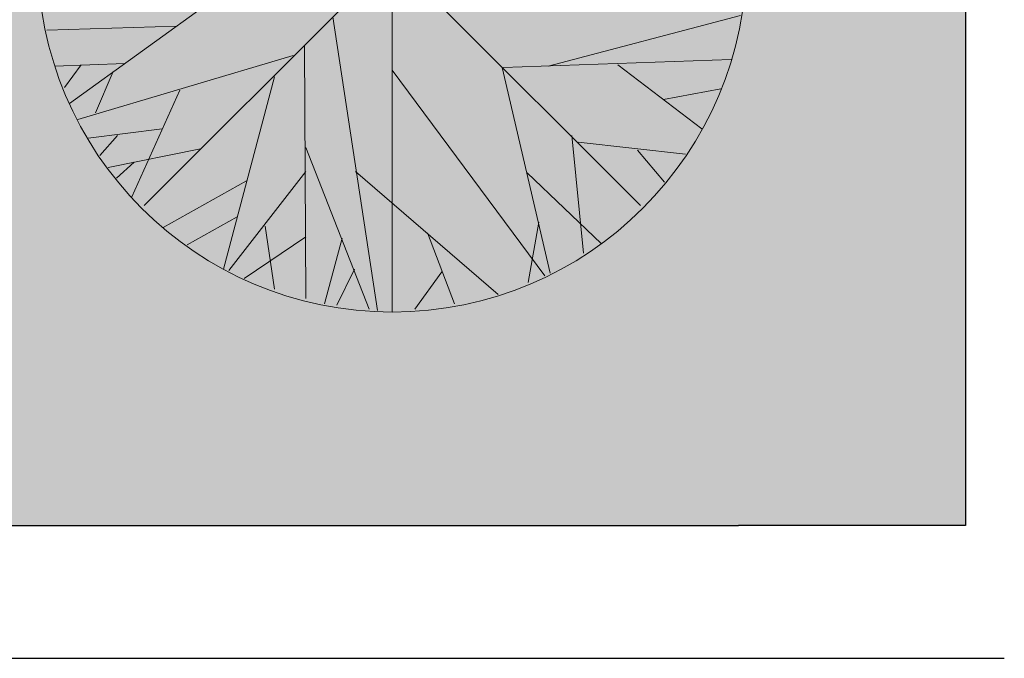
# Model space of a CAD drawing. Units: inches. Extents: x 459864 to 460310, y 324185 to 324787.
# Tile 73 of 112: x 460238 to 460271, y 324195 to 324217. Entities that reach past the tile are written whole.
import ezdxf

# ---------------------------------------------------------------- set-up
doc = ezdxf.new("R2010")
doc.units = ezdxf.units.IN
for name, color, linetype, lineweight in [('A-ANNO-DIMS', 2, 'Continuous', 18), ('C-PROP', 7, 'Continuous', 30), ('L-PLNT', 3, 'Continuous', 13), ('L-SITE-PATT', 252, 'Continuous', 13)]:
    doc.layers.add(name, color=color, linetype=linetype, lineweight=lineweight)
doc.styles.get("Standard").update_dxf_attribs({"font": 'arial.ttf'})
doc.dimstyles.new('ISO-25', dxfattribs={"dimtxt": 6, "dimasz": 2.5, "dimexe": 1.25, "dimexo": 0.625, "dimtad": 1, "dimdec": 1, "dimlunit": 3, "dimtxsty": 'Standard', "dimcen": 2.5, "dimadec": 0, "dimazin": 0, "dimtfac": 1, "dimtdec": 1, "dimtmove": 0, "dimatfit": 3, "dimfxl": 1, "dimarcsym": 0})

# ---------------------------------------------------------------- blocks, each defined once
blk = doc.blocks.new('Tree - deciduous plan')
for p, q in [((0, 59.9996), (0, -60)), ((42, 42), (-42, -42)), ((42, -42), (-42, 42)), ((-54.6162, -24.7335), (-20.2853, 0.0941)), ((26.3697, -18.4138), (58.9401, -9.8369)), ((-58.4895, -12.3197), (-36.4825, -11.6426)), ((-10.074, -10.0627), (-2.5036, -59.7178)), ((-53.2078, -27.442), (-16.7641, -16.6081)), ((-14.8275, -15.0282), (-14.6515, -57.6865)), ((-57.081, -18.4138), (-45.2853, -17.9624)), ((-52.6797, -18.188), (-55.4966, -22.0251)), ((18.7992, -18.6394), (57.3556, -17.2853)), ((38.1654, -18.188), (52.426, -29.0219)), ((-47.2219, -19.3166), (-50.2148, -26.3135)), ((-0.0388, -19.0909), (25.8415, -53.8495)), ((18.6232, -18.6394), (26.7218, -53.3981)), ((-19.9331, -20.2194), (-28.5599, -52.721)), ((-35.9543, -22.4765), (-44.0529, -40.5329)), ((45.9119, -24.0564), (55.595, -22.2508)), ((-38.9472, -29.0219), (-51.4472, -30.6018)), ((-46.5177, -30.1504), (-49.5106, -33.536)), ((30.419, -30.1504), (32.3556, -50.0125)), ((31.4753, -31.279), (49.6091, -33.3103)), ((-32.4331, -32.4075), (-48.1021, -35.5674)), ((-14.6515, -32.1818), (-3.912, -59.4922)), ((41.5105, -32.6332), (46.088, -38.0501)), ((-43.7008, -34.6645), (-46.6937, -37.373)), ((-14.6515, -36.2445), (-27.6797, -52.9467)), ((-6.2008, -36.2445), (17.919, -57.0094)), ((22.8485, -36.4702), (35.3485, -48.4326)), ((-24.6867, -37.8244), (-38.7712, -45.7241)), ((-26.2712, -43.9185), (-34.7219, -48.6583)), ((24.7852, -44.8213), (23.0246, -54.978)), ((-21.5177, -45.4984), (-19.9331, -56.1065)), ((5.9471, -46.6269), (10.5246, -58.5893)), ((-14.6515, -47.3041), (-25.0388, -54.3009)), ((-8.4895, -47.5298), (-11.4825, -58.5893)), ((-6.3768, -52.721), (-9.3698, -58.815)), ((8.4119, -53.1724), (3.8344, -59.4922))]:
    blk.add_line(p, q)
blk.add_circle((0, 0), 60)
blk = doc.blocks.new('*D65')
at = {"layer": 'A-ANNO-DIMS', "color": 0, "lineweight": -2, "transparency": 16777216}
for p, q in [((460247.74, 324283.483), (460302.765, 324283.483)), ((460301.515, 324280.983), (460301.515, 324197.483)), ((460271.74, 324194.983), (460302.765, 324194.983))]:
    blk.add_line(p, q, dxfattribs=at)
at = {"layer": 'A-ANNO-DIMS', "color": 0, "transparency": 16777216}
for points in [[(460301.098, 324280.983), (460301.932, 324280.983), (460301.515, 324283.483)], [(460301.098, 324197.483), (460301.932, 324197.483), (460301.515, 324194.983)]]:
    blk.add_solid(points, dxfattribs=at)
at = {"layer": 'Defpoints', "color": 0, "transparency": 16777216}
for p in [(460247.115, 324283.483), (460271.115, 324194.983), (460301.515, 324194.983)]:
    blk.add_point(p, dxfattribs=at)
at = {"layer": 'A-ANNO-DIMS', "color": 0, "transparency": 16777216, "insert": (460297.788, 324239.233), "char_height": 6, "attachment_point": 5, "rotation": 90}
blk.add_mtext('7\'-4 1/2"', dxfattribs=at)

msp = doc.modelspace()

# ---------------------------------------------------------------- hatches: boundary and pattern name
at = {"layer": 'L-SITE-PATT'}
h = msp.add_hatch(dxfattribs=at)
h.set_pattern_fill('DOTS', color=256)
h.paths.add_polyline_path([(460269.804, 324283.483), (460247.115, 324283.483), (460121.929, 324283.483), (460121.929, 324252.473), (460117.429, 324252.473), (460110.124, 324252.473), (460110.124, 324243.287), (460080.83, 324243.287), (460080.83, 324252.473), (460061.115, 324252.473), (460061.115, 324251.882), (460077.909, 324251.882), (460077.909, 324199.483), (460080.83, 324199.483), (460080.83, 324207.553), (460110.124, 324207.553), (460110.124, 324199.483), (460110.813, 324199.483), (460262.115, 324199.483), (460269.804, 324199.483)], flags=17)
edge = h.paths.add_edge_path(flags=0)
edge.add_ellipse((460222.59, 324263.813), major_axis=(-8.485, 8.485), ratio=1, start_angle=405, end_angle=495, ccw=False)
edge.add_line((460214.821, 324254.66), (460214.832, 324254.666))
edge.add_ellipse((460222.59, 324263.813), major_axis=(-8.485, 8.485), ratio=1, start_angle=405, end_angle=495, ccw=False)
edge.add_line((460210.759, 324261.781), (460210.768, 324261.787))
edge.add_ellipse((460222.59, 324263.813), major_axis=(-8.485, 8.485), ratio=1, start_angle=405, end_angle=495, ccw=False)
edge.add_ellipse((460222.59, 324263.813), major_axis=(-8.485, 8.485), ratio=1, start_angle=392.754, end_angle=405, ccw=False)
edge.add_ellipse((460222.59, 324263.813), major_axis=(-8.485, 8.485), ratio=1, start_angle=380.9347, end_angle=392.754, ccw=False)
edge.add_line((460211.337, 324267.985), (460211.34, 324267.985))
edge.add_ellipse((460222.59, 324263.813), major_axis=(-8.485, 8.485), ratio=1, start_angle=380.9347, end_angle=392.754, ccw=False)
edge.add_ellipse((460222.59, 324263.813), major_axis=(-8.485, 8.485), ratio=1, start_angle=347.9015, end_angle=380.9347, ccw=False)
edge.add_ellipse((460222.59, 324263.813), major_axis=(-8.485, 8.485), ratio=1, start_angle=327.0619, end_angle=347.9015, ccw=False)
edge.add_ellipse((460222.59, 324263.813), major_axis=(-8.485, 8.485), ratio=1, start_angle=278.3246, end_angle=327.0619, ccw=False)
edge.add_line((460225.158, 324275.536), (460225.158, 324275.535))
edge.add_ellipse((460222.59, 324263.813), major_axis=(-8.485, 8.485), ratio=1, start_angle=278.3246, end_angle=327.0619, ccw=False)
edge.add_ellipse((460222.59, 324263.813), major_axis=(-8.485, 8.485), ratio=1, start_angle=260.6436, end_angle=278.3246, ccw=False)
edge.add_ellipse((460222.59, 324263.813), major_axis=(-8.485, 8.485), ratio=1, start_angle=225, end_angle=260.6436, ccw=False)
edge.add_line((460234.509, 324265.243), (460234.501, 324265.239))
edge.add_ellipse((460222.59, 324263.813), major_axis=(-8.485, 8.485), ratio=1, start_angle=225, end_angle=260.6436, ccw=False)
edge.add_ellipse((460222.59, 324263.813), major_axis=(-8.485, 8.485), ratio=1, start_angle=495, end_angle=585, ccw=False)
edge.add_line((460234.437, 324261.861), (460234.424, 324261.858))
edge.add_ellipse((460222.59, 324263.813), major_axis=(-8.485, 8.485), ratio=1, start_angle=495, end_angle=585, ccw=False)
edge.add_line((460227.95, 324253.067), (460227.946, 324253.083))
edge.add_ellipse((460222.59, 324263.813), major_axis=(-8.485, 8.485), ratio=1, start_angle=495, end_angle=585, ccw=False)
edge.add_line((460226.223, 324252.369), (460226.211, 324252.38))
edge.add_ellipse((460222.59, 324263.813), major_axis=(-8.485, 8.485), ratio=1, start_angle=495, end_angle=585, ccw=False)
h.paths.add_polyline_path([(460219.651, 324254.347), (460218.461, 324253.545), (460218.275, 324254.789), (460219.642, 324256.542), (460219.625, 324260.848), (460216.11, 324257.333), (460214.35, 324256.978), (460215.416, 324259.356), (460212.524, 324258.496), (460213.137, 324259.93), (460218.507, 324263.813), (460222.59, 324263.813), (460222.59, 324267.807), (460218.176, 324272.212), (460219.026, 324274.639), (460222.59, 324272.811), (460222.59, 324275.423), (460223.057, 324274.825), (460222.675, 324273.492), (460225.912, 324267.135), (460219.625, 324260.848)], flags=0)
edge = h.paths.add_edge_path(flags=0)
edge.add_ellipse((460194.576, 324264.046), major_axis=(-8.485, 8.485), ratio=1, start_angle=495, end_angle=585, ccw=False)
edge.add_line((460199.936, 324253.3), (460199.932, 324253.316))
edge.add_ellipse((460194.576, 324264.046), major_axis=(-8.485, 8.485), ratio=1, start_angle=495, end_angle=585, ccw=False)
edge.add_line((460198.208, 324252.603), (460198.196, 324252.613))
edge.add_ellipse((460194.576, 324264.046), major_axis=(-8.485, 8.485), ratio=1, start_angle=495, end_angle=585, ccw=False)
edge.add_ellipse((460194.576, 324264.046), major_axis=(-8.485, 8.485), ratio=1, start_angle=405, end_angle=495, ccw=False)
edge.add_line((460186.806, 324254.893), (460186.817, 324254.899))
edge.add_ellipse((460194.576, 324264.046), major_axis=(-8.485, 8.485), ratio=1, start_angle=405, end_angle=495, ccw=False)
edge.add_line((460182.744, 324262.014), (460182.753, 324262.02))
edge.add_ellipse((460194.576, 324264.046), major_axis=(-8.485, 8.485), ratio=1, start_angle=405, end_angle=495, ccw=False)
edge.add_ellipse((460194.576, 324264.046), major_axis=(-8.485, 8.485), ratio=1, start_angle=392.754, end_angle=405, ccw=False)
edge.add_ellipse((460194.576, 324264.046), major_axis=(-8.485, 8.485), ratio=1, start_angle=380.9347, end_angle=392.754, ccw=False)
edge.add_line((460183.323, 324268.218), (460183.326, 324268.218))
edge.add_ellipse((460194.576, 324264.046), major_axis=(-8.485, 8.485), ratio=1, start_angle=380.9347, end_angle=392.754, ccw=False)
edge.add_ellipse((460194.576, 324264.046), major_axis=(-8.485, 8.485), ratio=1, start_angle=347.9015, end_angle=380.9347, ccw=False)
edge.add_ellipse((460194.576, 324264.046), major_axis=(-8.485, 8.485), ratio=1, start_angle=327.0619, end_angle=347.9015, ccw=False)
edge.add_ellipse((460194.576, 324264.046), major_axis=(-8.485, 8.485), ratio=1, start_angle=278.3246, end_angle=327.0619, ccw=False)
edge.add_line((460197.144, 324275.769), (460197.143, 324275.768))
edge.add_ellipse((460194.576, 324264.046), major_axis=(-8.485, 8.485), ratio=1, start_angle=278.3246, end_angle=327.0619, ccw=False)
edge.add_ellipse((460194.576, 324264.046), major_axis=(-8.485, 8.485), ratio=1, start_angle=260.6436, end_angle=278.3246, ccw=False)
edge.add_ellipse((460194.576, 324264.046), major_axis=(-8.485, 8.485), ratio=1, start_angle=225, end_angle=260.6436, ccw=False)
edge.add_line((460206.494, 324265.476), (460206.487, 324265.473))
edge.add_ellipse((460194.576, 324264.046), major_axis=(-8.485, 8.485), ratio=1, start_angle=225, end_angle=260.6436, ccw=False)
edge.add_ellipse((460194.576, 324264.046), major_axis=(-8.485, 8.485), ratio=1, start_angle=495, end_angle=585, ccw=False)
edge.add_line((460206.422, 324262.094), (460206.409, 324262.091))
h.paths.add_polyline_path([(460191.61, 324261.081), (460191.637, 324254.58), (460190.447, 324253.778), (460190.261, 324255.023), (460191.628, 324256.775), (460191.61, 324261.081), (460188.096, 324257.566), (460186.335, 324257.211), (460187.402, 324259.589), (460184.509, 324258.729), (460185.123, 324260.163), (460190.493, 324264.046), (460194.576, 324264.046), (460194.576, 324268.04), (460190.161, 324272.446), (460191.011, 324274.872), (460194.576, 324273.044), (460194.576, 324275.657), (460195.043, 324275.058), (460194.661, 324273.725), (460197.897, 324267.368)], flags=0)
edge = h.paths.add_edge_path(flags=0)
edge.add_ellipse((460252.912, 324263.578), major_axis=(-8.485, 8.485), ratio=1, start_angle=405, end_angle=495, ccw=False)
edge.add_line((460241.081, 324261.545), (460241.089, 324261.551))
edge.add_ellipse((460252.912, 324263.578), major_axis=(-8.485, 8.485), ratio=1, start_angle=405, end_angle=495, ccw=False)
edge.add_ellipse((460252.912, 324263.578), major_axis=(-8.485, 8.485), ratio=1, start_angle=392.754, end_angle=405, ccw=False)
edge.add_ellipse((460252.912, 324263.578), major_axis=(-8.485, 8.485), ratio=1, start_angle=380.9347, end_angle=392.754, ccw=False)
edge.add_line((460241.659, 324267.749), (460241.662, 324267.749))
edge.add_ellipse((460252.912, 324263.578), major_axis=(-8.485, 8.485), ratio=1, start_angle=380.9347, end_angle=392.754, ccw=False)
edge.add_ellipse((460252.912, 324263.578), major_axis=(-8.485, 8.485), ratio=1, start_angle=347.9015, end_angle=380.9347, ccw=False)
edge.add_ellipse((460252.912, 324263.578), major_axis=(-8.485, 8.485), ratio=1, start_angle=327.0619, end_angle=347.9015, ccw=False)
edge.add_ellipse((460252.912, 324263.578), major_axis=(-8.485, 8.485), ratio=1, start_angle=278.3246, end_angle=327.0619, ccw=False)
edge.add_line((460255.48, 324275.3), (460255.479, 324275.299))
edge.add_ellipse((460252.912, 324263.578), major_axis=(-8.485, 8.485), ratio=1, start_angle=278.3246, end_angle=327.0619, ccw=False)
edge.add_ellipse((460252.912, 324263.578), major_axis=(-8.485, 8.485), ratio=1, start_angle=260.6436, end_angle=278.3246, ccw=False)
edge.add_ellipse((460252.912, 324263.578), major_axis=(-8.485, 8.485), ratio=1, start_angle=225, end_angle=260.6436, ccw=False)
edge.add_line((460264.83, 324265.007), (460264.823, 324265.004))
edge.add_ellipse((460252.912, 324263.578), major_axis=(-8.485, 8.485), ratio=1, start_angle=225, end_angle=260.6436, ccw=False)
edge.add_ellipse((460252.912, 324263.578), major_axis=(-8.485, 8.485), ratio=1, start_angle=495, end_angle=585, ccw=False)
edge.add_line((460264.758, 324261.626), (460264.745, 324261.622))
edge.add_ellipse((460252.912, 324263.578), major_axis=(-8.485, 8.485), ratio=1, start_angle=495, end_angle=585, ccw=False)
edge.add_line((460258.272, 324252.832), (460258.268, 324252.848))
edge.add_ellipse((460252.912, 324263.578), major_axis=(-8.485, 8.485), ratio=1, start_angle=495, end_angle=585, ccw=False)
edge.add_line((460256.545, 324252.134), (460256.533, 324252.144))
edge.add_ellipse((460252.912, 324263.578), major_axis=(-8.485, 8.485), ratio=1, start_angle=495, end_angle=585, ccw=False)
edge.add_ellipse((460252.912, 324263.578), major_axis=(-8.485, 8.485), ratio=1, start_angle=405, end_angle=495, ccw=False)
edge.add_line((460245.143, 324254.424), (460245.153, 324254.43))
h.paths.add_polyline_path([(460244.672, 324256.742), (460245.738, 324259.12), (460242.846, 324258.26), (460243.459, 324259.694), (460248.829, 324263.578), (460252.912, 324263.578), (460252.912, 324267.571), (460248.497, 324271.977), (460249.348, 324274.403), (460252.912, 324272.576), (460252.912, 324275.188), (460253.379, 324274.589), (460252.997, 324273.257), (460256.233, 324266.899), (460249.946, 324260.612), (460249.973, 324254.111), (460248.783, 324253.309), (460248.597, 324254.554), (460249.964, 324256.306), (460249.946, 324260.612), (460246.432, 324257.097)], flags=0)
edge = h.paths.add_edge_path(flags=0)
edge.add_ellipse((460167.439, 324262.833), major_axis=(-8.485, 8.485), ratio=1, start_angle=495, end_angle=585, ccw=False)
edge.add_line((460172.799, 324252.087), (460172.795, 324252.103))
edge.add_ellipse((460167.439, 324262.833), major_axis=(-8.485, 8.485), ratio=1, start_angle=495, end_angle=585, ccw=False)
edge.add_line((460171.071, 324251.389), (460171.059, 324251.399))
edge.add_ellipse((460167.439, 324262.833), major_axis=(-8.485, 8.485), ratio=1, start_angle=495, end_angle=585, ccw=False)
edge.add_ellipse((460167.439, 324262.833), major_axis=(-8.485, 8.485), ratio=1, start_angle=405, end_angle=495, ccw=False)
edge.add_line((460159.669, 324253.679), (460159.68, 324253.685))
edge.add_ellipse((460167.439, 324262.833), major_axis=(-8.485, 8.485), ratio=1, start_angle=405, end_angle=495, ccw=False)
edge.add_line((460155.607, 324260.8), (460155.616, 324260.806))
edge.add_ellipse((460167.439, 324262.833), major_axis=(-8.485, 8.485), ratio=1, start_angle=405, end_angle=495, ccw=False)
edge.add_ellipse((460167.439, 324262.833), major_axis=(-8.485, 8.485), ratio=1, start_angle=392.754, end_angle=405, ccw=False)
edge.add_ellipse((460167.439, 324262.833), major_axis=(-8.485, 8.485), ratio=1, start_angle=380.9347, end_angle=392.754, ccw=False)
edge.add_line((460156.185, 324267.005), (460156.189, 324267.005))
edge.add_ellipse((460167.439, 324262.833), major_axis=(-8.485, 8.485), ratio=1, start_angle=380.9347, end_angle=392.754, ccw=False)
edge.add_ellipse((460167.439, 324262.833), major_axis=(-8.485, 8.485), ratio=1, start_angle=347.9015, end_angle=380.9347, ccw=False)
edge.add_ellipse((460167.439, 324262.833), major_axis=(-8.485, 8.485), ratio=1, start_angle=327.0619, end_angle=347.9015, ccw=False)
edge.add_ellipse((460167.439, 324262.833), major_axis=(-8.485, 8.485), ratio=1, start_angle=278.3246, end_angle=327.0619, ccw=False)
edge.add_line((460170.007, 324274.556), (460170.006, 324274.554))
edge.add_ellipse((460167.439, 324262.833), major_axis=(-8.485, 8.485), ratio=1, start_angle=278.3246, end_angle=327.0619, ccw=False)
edge.add_ellipse((460167.439, 324262.833), major_axis=(-8.485, 8.485), ratio=1, start_angle=260.6436, end_angle=278.3246, ccw=False)
edge.add_ellipse((460167.439, 324262.833), major_axis=(-8.485, 8.485), ratio=1, start_angle=225, end_angle=260.6436, ccw=False)
edge.add_line((460179.357, 324264.262), (460179.35, 324264.259))
edge.add_ellipse((460167.439, 324262.833), major_axis=(-8.485, 8.485), ratio=1, start_angle=225, end_angle=260.6436, ccw=False)
edge.add_ellipse((460167.439, 324262.833), major_axis=(-8.485, 8.485), ratio=1, start_angle=495, end_angle=585, ccw=False)
edge.add_line((460179.285, 324260.881), (460179.272, 324260.877))
h.paths.add_polyline_path([(460164.473, 324259.867), (460164.5, 324253.366), (460163.31, 324252.565), (460163.124, 324253.809), (460164.491, 324255.561), (460164.473, 324259.867), (460160.958, 324256.353), (460159.198, 324255.998), (460160.265, 324258.375), (460157.372, 324257.515), (460157.986, 324258.949), (460163.356, 324262.833), (460167.439, 324262.833), (460167.439, 324266.826), (460163.024, 324271.232), (460163.874, 324273.659), (460167.439, 324271.831), (460167.439, 324274.443), (460167.905, 324273.844), (460167.524, 324272.512), (460170.76, 324266.154)], flags=0)
edge = h.paths.add_edge_path(flags=0)
edge.add_ellipse((460140.758, 324262.37), major_axis=(-8.485, 8.485), ratio=1, start_angle=495, end_angle=585, ccw=False)
edge.add_line((460146.118, 324251.624), (460146.114, 324251.639))
edge.add_ellipse((460140.758, 324262.37), major_axis=(-8.485, 8.485), ratio=1, start_angle=495, end_angle=585, ccw=False)
edge.add_line((460144.391, 324250.926), (460144.379, 324250.936))
edge.add_ellipse((460140.758, 324262.37), major_axis=(-8.485, 8.485), ratio=1, start_angle=495, end_angle=585, ccw=False)
edge.add_ellipse((460140.758, 324262.37), major_axis=(-8.485, 8.485), ratio=1, start_angle=405, end_angle=495, ccw=False)
edge.add_line((460132.989, 324253.216), (460132.999, 324253.222))
edge.add_ellipse((460140.758, 324262.37), major_axis=(-8.485, 8.485), ratio=1, start_angle=405, end_angle=495, ccw=False)
edge.add_line((460128.927, 324260.337), (460128.935, 324260.343))
edge.add_ellipse((460140.758, 324262.37), major_axis=(-8.485, 8.485), ratio=1, start_angle=405, end_angle=495, ccw=False)
edge.add_ellipse((460140.758, 324262.37), major_axis=(-8.485, 8.485), ratio=1, start_angle=392.754, end_angle=405, ccw=False)
edge.add_ellipse((460140.758, 324262.37), major_axis=(-8.485, 8.485), ratio=1, start_angle=380.9347, end_angle=392.754, ccw=False)
edge.add_line((460129.505, 324266.541), (460129.508, 324266.541))
edge.add_ellipse((460140.758, 324262.37), major_axis=(-8.485, 8.485), ratio=1, start_angle=380.9347, end_angle=392.754, ccw=False)
edge.add_ellipse((460140.758, 324262.37), major_axis=(-8.485, 8.485), ratio=1, start_angle=347.9015, end_angle=380.9347, ccw=False)
edge.add_ellipse((460140.758, 324262.37), major_axis=(-8.485, 8.485), ratio=1, start_angle=327.0619, end_angle=347.9015, ccw=False)
edge.add_ellipse((460140.758, 324262.37), major_axis=(-8.485, 8.485), ratio=1, start_angle=278.3246, end_angle=327.0619, ccw=False)
edge.add_line((460143.326, 324274.092), (460143.325, 324274.091))
edge.add_ellipse((460140.758, 324262.37), major_axis=(-8.485, 8.485), ratio=1, start_angle=278.3246, end_angle=327.0619, ccw=False)
edge.add_ellipse((460140.758, 324262.37), major_axis=(-8.485, 8.485), ratio=1, start_angle=260.6436, end_angle=278.3246, ccw=False)
edge.add_ellipse((460140.758, 324262.37), major_axis=(-8.485, 8.485), ratio=1, start_angle=225, end_angle=260.6436, ccw=False)
edge.add_line((460152.677, 324263.799), (460152.669, 324263.796))
edge.add_ellipse((460140.758, 324262.37), major_axis=(-8.485, 8.485), ratio=1, start_angle=225, end_angle=260.6436, ccw=False)
edge.add_ellipse((460140.758, 324262.37), major_axis=(-8.485, 8.485), ratio=1, start_angle=495, end_angle=585, ccw=False)
edge.add_line((460152.604, 324260.418), (460152.592, 324260.414))
h.paths.add_polyline_path([(460137.792, 324259.404), (460137.819, 324252.903), (460136.629, 324252.101), (460136.443, 324253.346), (460137.81, 324255.098), (460137.792, 324259.404), (460134.278, 324255.889), (460132.518, 324255.534), (460133.584, 324257.912), (460130.692, 324257.052), (460131.305, 324258.486), (460136.675, 324262.37), (460140.758, 324262.37), (460140.758, 324266.363), (460136.343, 324270.769), (460137.194, 324273.195), (460140.758, 324271.367), (460140.758, 324273.98), (460141.225, 324273.381), (460140.843, 324272.049), (460144.079, 324265.691)], flags=0)
h.paths.add_polyline_path([(460110.124, 324227.414), (460080.83, 324227.414), (460080.83, 324235.484), (460110.124, 324235.484)], flags=16)
h.paths.add_polyline_path([(460110.124, 324220.797), (460110.124, 324212.727), (460080.83, 324212.727), (460080.83, 324220.797)], flags=16)
h.paths.add_polyline_path([(460269.804, 324283.483), (460247.115, 324283.483), (460121.929, 324283.483), (460121.929, 324252.473), (460117.429, 324252.473), (460110.124, 324252.473), (460110.124, 324243.287), (460080.83, 324243.287), (460080.83, 324252.473), (460061.115, 324252.473), (460061.115, 324251.882), (460077.909, 324251.882), (460077.909, 324199.483), (460080.83, 324199.483), (460080.83, 324207.553), (460110.124, 324207.553), (460110.124, 324199.483), (460262.115, 324199.483), (460269.804, 324199.483)], flags=17)
h.paths.add_polyline_path([(460219.651, 324254.347), (460218.461, 324253.545), (460218.275, 324254.789), (460219.642, 324256.542), (460219.625, 324260.848), (460216.11, 324257.333), (460214.35, 324256.978), (460215.416, 324259.356), (460212.524, 324258.496), (460213.137, 324259.93), (460218.507, 324263.813), (460222.59, 324263.813), (460220.18, 324266.223), (460215.461, 324265.308), (460211.835, 324266.137), (460216.247, 324267.985), (460218.418, 324267.985), (460222.59, 324263.813), (460222.59, 324267.807), (460218.176, 324272.212), (460219.026, 324274.639), (460222.59, 324272.811), (460222.59, 324275.423), (460223.057, 324274.825), (460222.675, 324273.492), (460225.912, 324267.135), (460222.59, 324263.813), (460231.383, 324263.813), (460228.485, 324262.488), (460224.425, 324261.978), (460228.68, 324257.724), (460228.966, 324254.791), (460227.142, 324256.537), (460227.542, 324254.819), (460227.333, 324253.614), (460222.59, 324259.985), (460222.59, 324255.497), (460221.377, 324256.541), (460220.576, 324261.799), (460219.625, 324260.848)], flags=0)
h.paths.add_polyline_path([(460199.127, 324256.77), (460199.528, 324255.052), (460199.319, 324253.848), (460194.576, 324260.218), (460194.576, 324255.73), (460193.363, 324256.774), (460192.561, 324262.032), (460191.61, 324261.081), (460191.637, 324254.58), (460190.447, 324253.778), (460190.261, 324255.023), (460191.628, 324256.775), (460191.61, 324261.081), (460188.096, 324257.566), (460186.335, 324257.211), (460187.402, 324259.589), (460184.509, 324258.729), (460185.123, 324260.163), (460190.493, 324264.046), (460194.576, 324264.046), (460192.166, 324266.456), (460187.446, 324265.541), (460183.82, 324266.37), (460188.232, 324268.218), (460190.404, 324268.218), (460194.576, 324264.046), (460194.576, 324268.04), (460190.161, 324272.446), (460191.011, 324274.872), (460194.576, 324273.044), (460194.576, 324275.657), (460195.043, 324275.058), (460194.661, 324273.725), (460197.897, 324267.368), (460194.576, 324264.046), (460203.368, 324264.046), (460200.47, 324262.721), (460196.411, 324262.212), (460200.665, 324257.957), (460200.951, 324255.024)], flags=0)
h.paths.add_polyline_path([(460244.672, 324256.742), (460245.738, 324259.12), (460242.846, 324258.26), (460243.459, 324259.694), (460248.829, 324263.578), (460252.912, 324263.578), (460250.502, 324265.987), (460245.783, 324265.072), (460242.156, 324265.901), (460246.568, 324267.749), (460248.74, 324267.749), (460252.912, 324263.578), (460252.912, 324267.571), (460248.497, 324271.977), (460249.348, 324274.403), (460252.912, 324272.576), (460252.912, 324275.188), (460253.379, 324274.589), (460252.997, 324273.257), (460256.233, 324266.899), (460252.912, 324263.578), (460261.705, 324263.578), (460258.806, 324262.252), (460254.747, 324261.743), (460259.002, 324257.488), (460259.288, 324254.555), (460257.463, 324256.301), (460257.864, 324254.583), (460257.655, 324253.379), (460252.912, 324259.749), (460252.912, 324255.261), (460251.699, 324256.305), (460250.897, 324261.563), (460249.946, 324260.612), (460249.973, 324254.111), (460248.783, 324253.309), (460248.597, 324254.554), (460249.964, 324256.306), (460249.946, 324260.612), (460246.432, 324257.097)], flags=0)
h.paths.add_polyline_path([(460173.528, 324256.743), (460173.814, 324253.811), (460171.99, 324255.556), (460172.39, 324253.838), (460172.182, 324252.634), (460167.439, 324259.004), (460167.439, 324254.516), (460166.226, 324255.56), (460165.424, 324260.818), (460164.473, 324259.867), (460164.5, 324253.366), (460163.31, 324252.565), (460163.124, 324253.809), (460164.491, 324255.561), (460164.473, 324259.867), (460160.958, 324256.353), (460159.198, 324255.998), (460160.265, 324258.375), (460157.372, 324257.515), (460157.986, 324258.949), (460163.356, 324262.833), (460167.439, 324262.833), (460165.029, 324265.243), (460160.309, 324264.327), (460156.683, 324265.156), (460161.095, 324267.005), (460163.267, 324267.005), (460167.439, 324262.833), (460167.439, 324266.826), (460163.024, 324271.232), (460163.874, 324273.659), (460167.439, 324271.831), (460167.439, 324274.443), (460167.905, 324273.844), (460167.524, 324272.512), (460170.76, 324266.154), (460167.439, 324262.833), (460176.231, 324262.833), (460173.333, 324261.507), (460169.274, 324260.998)], flags=0)
h.paths.add_polyline_path([(460146.848, 324256.28), (460147.134, 324253.347), (460145.31, 324255.093), (460145.71, 324253.375), (460145.501, 324252.171), (460140.758, 324258.541), (460140.758, 324254.053), (460139.545, 324255.097), (460138.744, 324260.355), (460137.792, 324259.404), (460137.819, 324252.903), (460136.629, 324252.101), (460136.443, 324253.346), (460137.81, 324255.098), (460137.792, 324259.404), (460134.278, 324255.889), (460132.518, 324255.534), (460133.584, 324257.912), (460130.692, 324257.052), (460131.305, 324258.486), (460136.675, 324262.37), (460140.758, 324262.37), (460138.348, 324264.779), (460133.629, 324263.864), (460130.002, 324264.693), (460134.414, 324266.541), (460136.586, 324266.541), (460140.758, 324262.37), (460140.758, 324266.363), (460136.343, 324270.769), (460137.194, 324273.195), (460140.758, 324271.367), (460140.758, 324273.98), (460141.225, 324273.381), (460140.843, 324272.049), (460144.079, 324265.691), (460140.758, 324262.37), (460149.551, 324262.37), (460146.653, 324261.044), (460142.593, 324260.535)], flags=0)
edge = h.paths.add_edge_path()
edge.add_line((460269.804, 324272.549), (460260.881, 324272.549))
edge.add_ellipse((460252.912, 324263.578), major_axis=(-8.485, 8.485), ratio=1, start_angle=260.6436, end_angle=273.3846, ccw=False)
edge.add_line((460262.283, 324271.092), (460262.261, 324271.091))
edge.add_ellipse((460252.912, 324263.578), major_axis=(-8.485, 8.485), ratio=1, start_angle=260.6436, end_angle=273.3846, ccw=False)
edge.add_ellipse((460252.912, 324263.578), major_axis=(-8.485, 8.485), ratio=1, start_angle=225, end_angle=260.6436, ccw=False)
edge.add_line((460263.609, 324269.063), (460263.572, 324269.058))
edge.add_ellipse((460252.912, 324263.578), major_axis=(-8.485, 8.485), ratio=1, start_angle=225, end_angle=260.6436, ccw=False)
edge.add_line((460264.615, 324266.306), (460264.585, 324266.305))
edge.add_ellipse((460252.912, 324263.578), major_axis=(-8.485, 8.485), ratio=1, start_angle=225, end_angle=260.6436, ccw=False)
edge.add_line((460264.83, 324265.007), (460264.823, 324265.004))
edge.add_ellipse((460252.912, 324263.578), major_axis=(-8.485, 8.485), ratio=1, start_angle=225, end_angle=260.6436, ccw=False)
edge.add_ellipse((460252.912, 324263.578), major_axis=(-8.485, 8.485), ratio=1, start_angle=495, end_angle=585, ccw=False)
edge.add_line((460264.758, 324261.626), (460264.745, 324261.622))
edge.add_ellipse((460252.912, 324263.578), major_axis=(-8.485, 8.485), ratio=1, start_angle=495, end_angle=585, ccw=False)
edge.add_line((460263.442, 324257.739), (460263.389, 324257.779))
edge.add_ellipse((460252.912, 324263.578), major_axis=(-8.485, 8.485), ratio=1, start_angle=495, end_angle=585, ccw=False)
edge.add_line((460258.128, 324252.744), (460258.102, 324252.779))
edge.add_ellipse((460252.912, 324263.578), major_axis=(-8.485, 8.485), ratio=1, start_angle=495, end_angle=585, ccw=False)
edge.add_line((460256.545, 324252.134), (460256.533, 324252.144))
edge.add_ellipse((460252.912, 324263.578), major_axis=(-8.485, 8.485), ratio=1, start_angle=495, end_angle=585, ccw=False)
edge.add_ellipse((460252.912, 324263.578), major_axis=(-8.485, 8.485), ratio=1, start_angle=405, end_angle=495, ccw=False)
edge.add_line((460250.594, 324251.78), (460250.605, 324251.82))
edge.add_ellipse((460252.912, 324263.578), major_axis=(-8.485, 8.485), ratio=1, start_angle=405, end_angle=495, ccw=False)
edge.add_line((460245.143, 324254.424), (460245.153, 324254.43))
edge.add_ellipse((460252.912, 324263.578), major_axis=(-8.485, 8.485), ratio=1, start_angle=405, end_angle=495, ccw=False)
edge.add_line((460243.525, 324256.059), (460243.56, 324256.091))
edge.add_ellipse((460252.912, 324263.578), major_axis=(-8.485, 8.485), ratio=1, start_angle=405, end_angle=495, ccw=False)
edge.add_line((460241.44, 324259.893), (460241.522, 324259.896))
edge.add_ellipse((460252.912, 324263.578), major_axis=(-8.485, 8.485), ratio=1, start_angle=405, end_angle=495, ccw=False)
edge.add_line((460241.081, 324261.545), (460241.089, 324261.551))
edge.add_ellipse((460252.912, 324263.578), major_axis=(-8.485, 8.485), ratio=1, start_angle=405, end_angle=495, ccw=False)
edge.add_ellipse((460252.912, 324263.578), major_axis=(-8.485, 8.485), ratio=1, start_angle=392.754, end_angle=405, ccw=False)
edge.add_line((460241.05, 324265.438), (460241.063, 324265.443))
edge.add_ellipse((460252.912, 324263.578), major_axis=(-8.485, 8.485), ratio=1, start_angle=392.754, end_angle=405, ccw=False)
edge.add_ellipse((460252.912, 324263.578), major_axis=(-8.485, 8.485), ratio=1, start_angle=380.9347, end_angle=392.754, ccw=False)
edge.add_line((460241.452, 324267.176), (460241.469, 324267.171))
edge.add_ellipse((460252.912, 324263.578), major_axis=(-8.485, 8.485), ratio=1, start_angle=380.9347, end_angle=392.754, ccw=False)
edge.add_line((460241.659, 324267.749), (460241.662, 324267.749))
edge.add_ellipse((460252.912, 324263.578), major_axis=(-8.485, 8.485), ratio=1, start_angle=380.9347, end_angle=392.754, ccw=False)
edge.add_ellipse((460252.912, 324263.578), major_axis=(-8.485, 8.485), ratio=1, start_angle=356.6154, end_angle=380.9347, ccw=False)
edge.add_line((460244.88, 324272.488), (460244.713, 324272.549))
edge.add_line((460244.713, 324272.549), (460230.817, 324272.549))
edge.add_ellipse((460222.59, 324263.813), major_axis=(-8.485, 8.485), ratio=1, start_angle=260.6436, end_angle=271.7178, ccw=False)
edge.add_ellipse((460222.59, 324263.813), major_axis=(-8.485, 8.485), ratio=1, start_angle=225, end_angle=260.6436, ccw=False)
edge.add_line((460233.287, 324269.299), (460233.25, 324269.294))
edge.add_ellipse((460222.59, 324263.813), major_axis=(-8.485, 8.485), ratio=1, start_angle=225, end_angle=260.6436, ccw=False)
edge.add_line((460234.294, 324266.541), (460234.264, 324266.541))
edge.add_ellipse((460222.59, 324263.813), major_axis=(-8.485, 8.485), ratio=1, start_angle=225, end_angle=260.6436, ccw=False)
edge.add_line((460234.509, 324265.243), (460234.501, 324265.239))
edge.add_ellipse((460222.59, 324263.813), major_axis=(-8.485, 8.485), ratio=1, start_angle=225, end_angle=260.6436, ccw=False)
edge.add_ellipse((460222.59, 324263.813), major_axis=(-8.485, 8.485), ratio=1, start_angle=495, end_angle=585, ccw=False)
edge.add_line((460234.437, 324261.861), (460234.424, 324261.858))
edge.add_ellipse((460222.59, 324263.813), major_axis=(-8.485, 8.485), ratio=1, start_angle=495, end_angle=585, ccw=False)
edge.add_line((460233.121, 324257.975), (460233.068, 324258.015))
edge.add_ellipse((460222.59, 324263.813), major_axis=(-8.485, 8.485), ratio=1, start_angle=495, end_angle=585, ccw=False)
edge.add_line((460227.806, 324252.979), (460227.78, 324253.014))
edge.add_ellipse((460222.59, 324263.813), major_axis=(-8.485, 8.485), ratio=1, start_angle=495, end_angle=585, ccw=False)
edge.add_line((460226.223, 324252.369), (460226.211, 324252.38))
edge.add_ellipse((460222.59, 324263.813), major_axis=(-8.485, 8.485), ratio=1, start_angle=495, end_angle=585, ccw=False)
edge.add_ellipse((460222.59, 324263.813), major_axis=(-8.485, 8.485), ratio=1, start_angle=405, end_angle=495, ccw=False)
edge.add_line((460220.272, 324252.016), (460220.283, 324252.055))
edge.add_ellipse((460222.59, 324263.813), major_axis=(-8.485, 8.485), ratio=1, start_angle=405, end_angle=495, ccw=False)
edge.add_line((460214.821, 324254.66), (460214.832, 324254.666))
edge.add_ellipse((460222.59, 324263.813), major_axis=(-8.485, 8.485), ratio=1, start_angle=405, end_angle=495, ccw=False)
edge.add_line((460213.203, 324256.295), (460213.239, 324256.327))
edge.add_ellipse((460222.59, 324263.813), major_axis=(-8.485, 8.485), ratio=1, start_angle=405, end_angle=495, ccw=False)
edge.add_line((460211.118, 324260.128), (460211.201, 324260.131))
edge.add_ellipse((460222.59, 324263.813), major_axis=(-8.485, 8.485), ratio=1, start_angle=405, end_angle=495, ccw=False)
edge.add_line((460210.759, 324261.781), (460210.768, 324261.787))
edge.add_ellipse((460222.59, 324263.813), major_axis=(-8.485, 8.485), ratio=1, start_angle=405, end_angle=495, ccw=False)
edge.add_ellipse((460222.59, 324263.813), major_axis=(-8.485, 8.485), ratio=1, start_angle=392.754, end_angle=405, ccw=False)
edge.add_line((460210.729, 324265.673), (460210.741, 324265.678))
edge.add_ellipse((460222.59, 324263.813), major_axis=(-8.485, 8.485), ratio=1, start_angle=392.754, end_angle=405, ccw=False)
edge.add_ellipse((460222.59, 324263.813), major_axis=(-8.485, 8.485), ratio=1, start_angle=380.9347, end_angle=392.754, ccw=False)
edge.add_line((460211.13, 324267.412), (460211.147, 324267.407))
edge.add_ellipse((460222.59, 324263.813), major_axis=(-8.485, 8.485), ratio=1, start_angle=380.9347, end_angle=392.754, ccw=False)
edge.add_line((460211.337, 324267.985), (460211.34, 324267.985))
edge.add_ellipse((460222.59, 324263.813), major_axis=(-8.485, 8.485), ratio=1, start_angle=380.9347, end_angle=392.754, ccw=False)
edge.add_ellipse((460222.59, 324263.813), major_axis=(-8.485, 8.485), ratio=1, start_angle=358.2822, end_angle=380.9347, ccw=False)
edge.add_line((460213.705, 324271.902), (460213.709, 324271.869))
edge.add_ellipse((460222.59, 324263.813), major_axis=(-8.485, 8.485), ratio=1, start_angle=358.2822, end_angle=380.9347, ccw=False)
edge.add_line((460214.363, 324272.549), (460203.078, 324272.549))
edge.add_line((460203.078, 324272.549), (460203.06, 324272.531))
edge.add_ellipse((460194.576, 324264.046), major_axis=(-8.485, 8.485), ratio=1, start_angle=260.6436, end_angle=270.1168, ccw=False)
edge.add_line((460203.957, 324271.561), (460203.921, 324271.56))
edge.add_ellipse((460194.576, 324264.046), major_axis=(-8.485, 8.485), ratio=1, start_angle=260.6436, end_angle=270.1168, ccw=False)
edge.add_ellipse((460194.576, 324264.046), major_axis=(-8.485, 8.485), ratio=1, start_angle=225, end_angle=260.6436, ccw=False)
edge.add_line((460205.272, 324269.532), (460205.235, 324269.527))
edge.add_ellipse((460194.576, 324264.046), major_axis=(-8.485, 8.485), ratio=1, start_angle=225, end_angle=260.6436, ccw=False)
edge.add_line((460206.279, 324266.774), (460206.249, 324266.774))
edge.add_ellipse((460194.576, 324264.046), major_axis=(-8.485, 8.485), ratio=1, start_angle=225, end_angle=260.6436, ccw=False)
edge.add_line((460206.494, 324265.476), (460206.487, 324265.473))
edge.add_ellipse((460194.576, 324264.046), major_axis=(-8.485, 8.485), ratio=1, start_angle=225, end_angle=260.6436, ccw=False)
edge.add_ellipse((460194.576, 324264.046), major_axis=(-8.485, 8.485), ratio=1, start_angle=495, end_angle=585, ccw=False)
edge.add_line((460206.422, 324262.094), (460206.409, 324262.091))
edge.add_ellipse((460194.576, 324264.046), major_axis=(-8.485, 8.485), ratio=1, start_angle=495, end_angle=585, ccw=False)
edge.add_line((460205.106, 324258.208), (460205.053, 324258.248))
edge.add_ellipse((460194.576, 324264.046), major_axis=(-8.485, 8.485), ratio=1, start_angle=495, end_angle=585, ccw=False)
edge.add_line((460199.792, 324253.212), (460199.766, 324253.248))
edge.add_ellipse((460194.576, 324264.046), major_axis=(-8.485, 8.485), ratio=1, start_angle=495, end_angle=585, ccw=False)
edge.add_line((460198.208, 324252.603), (460198.196, 324252.613))
edge.add_ellipse((460194.576, 324264.046), major_axis=(-8.485, 8.485), ratio=1, start_angle=495, end_angle=585, ccw=False)
edge.add_ellipse((460194.576, 324264.046), major_axis=(-8.485, 8.485), ratio=1, start_angle=405, end_angle=495, ccw=False)
edge.add_line((460192.258, 324252.249), (460192.268, 324252.289))
edge.add_ellipse((460194.576, 324264.046), major_axis=(-8.485, 8.485), ratio=1, start_angle=405, end_angle=495, ccw=False)
edge.add_line((460186.806, 324254.893), (460186.817, 324254.899))
edge.add_ellipse((460194.576, 324264.046), major_axis=(-8.485, 8.485), ratio=1, start_angle=405, end_angle=495, ccw=False)
edge.add_line((460185.188, 324256.528), (460185.224, 324256.56))
edge.add_ellipse((460194.576, 324264.046), major_axis=(-8.485, 8.485), ratio=1, start_angle=405, end_angle=495, ccw=False)
edge.add_line((460183.104, 324260.362), (460183.186, 324260.365))
edge.add_ellipse((460194.576, 324264.046), major_axis=(-8.485, 8.485), ratio=1, start_angle=405, end_angle=495, ccw=False)
edge.add_line((460182.744, 324262.014), (460182.753, 324262.02))
edge.add_ellipse((460194.576, 324264.046), major_axis=(-8.485, 8.485), ratio=1, start_angle=405, end_angle=495, ccw=False)
edge.add_ellipse((460194.576, 324264.046), major_axis=(-8.485, 8.485), ratio=1, start_angle=392.754, end_angle=405, ccw=False)
edge.add_line((460182.714, 324265.906), (460182.726, 324265.912))
edge.add_ellipse((460194.576, 324264.046), major_axis=(-8.485, 8.485), ratio=1, start_angle=392.754, end_angle=405, ccw=False)
edge.add_ellipse((460194.576, 324264.046), major_axis=(-8.485, 8.485), ratio=1, start_angle=380.9347, end_angle=392.754, ccw=False)
edge.add_line((460183.116, 324267.645), (460183.133, 324267.64))
edge.add_ellipse((460194.576, 324264.046), major_axis=(-8.485, 8.485), ratio=1, start_angle=380.9347, end_angle=392.754, ccw=False)
edge.add_line((460183.323, 324268.218), (460183.326, 324268.218))
edge.add_ellipse((460194.576, 324264.046), major_axis=(-8.485, 8.485), ratio=1, start_angle=380.9347, end_angle=392.754, ccw=False)
edge.add_ellipse((460194.576, 324264.046), major_axis=(-8.485, 8.485), ratio=1, start_angle=359.8832, end_angle=380.9347, ccw=False)
edge.add_line((460184.491, 324270.611), (460184.553, 324270.611))
edge.add_ellipse((460194.576, 324264.046), major_axis=(-8.485, 8.485), ratio=1, start_angle=359.8832, end_angle=380.9347, ccw=False)
edge.add_line((460185.346, 324271.76), (460185.379, 324271.728))
edge.add_ellipse((460194.576, 324264.046), major_axis=(-8.485, 8.485), ratio=1, start_angle=359.8832, end_angle=380.9347, ccw=False)
edge.add_line((460185.697, 324272.086), (460185.633, 324272.549))
edge.add_line((460185.633, 324272.549), (460174.683, 324272.549))
edge.add_line((460174.683, 324272.549), (460174.606, 324272.457))
edge.add_ellipse((460167.439, 324262.833), major_axis=(-8.485, 8.485), ratio=1, start_angle=260.6436, end_angle=278.3246, ccw=False)
edge.add_ellipse((460167.439, 324262.833), major_axis=(-8.485, 8.485), ratio=1, start_angle=225, end_angle=260.6436, ccw=False)
edge.add_line((460178.135, 324268.318), (460178.098, 324268.313))
edge.add_ellipse((460167.439, 324262.833), major_axis=(-8.485, 8.485), ratio=1, start_angle=225, end_angle=260.6436, ccw=False)
edge.add_line((460179.142, 324265.561), (460179.112, 324265.56))
edge.add_ellipse((460167.439, 324262.833), major_axis=(-8.485, 8.485), ratio=1, start_angle=225, end_angle=260.6436, ccw=False)
edge.add_line((460179.357, 324264.262), (460179.35, 324264.259))
edge.add_ellipse((460167.439, 324262.833), major_axis=(-8.485, 8.485), ratio=1, start_angle=225, end_angle=260.6436, ccw=False)
edge.add_ellipse((460167.439, 324262.833), major_axis=(-8.485, 8.485), ratio=1, start_angle=495, end_angle=585, ccw=False)
edge.add_line((460179.285, 324260.881), (460179.272, 324260.877))
edge.add_ellipse((460167.439, 324262.833), major_axis=(-8.485, 8.485), ratio=1, start_angle=495, end_angle=585, ccw=False)
edge.add_line((460177.969, 324256.994), (460177.916, 324257.034))
edge.add_ellipse((460167.439, 324262.833), major_axis=(-8.485, 8.485), ratio=1, start_angle=495, end_angle=585, ccw=False)
edge.add_line((460172.655, 324251.999), (460172.629, 324252.034))
edge.add_ellipse((460167.439, 324262.833), major_axis=(-8.485, 8.485), ratio=1, start_angle=495, end_angle=585, ccw=False)
edge.add_line((460171.071, 324251.389), (460171.059, 324251.399))
edge.add_ellipse((460167.439, 324262.833), major_axis=(-8.485, 8.485), ratio=1, start_angle=495, end_angle=585, ccw=False)
edge.add_ellipse((460167.439, 324262.833), major_axis=(-8.485, 8.485), ratio=1, start_angle=405, end_angle=495, ccw=False)
edge.add_line((460165.121, 324251.036), (460165.131, 324251.075))
edge.add_ellipse((460167.439, 324262.833), major_axis=(-8.485, 8.485), ratio=1, start_angle=405, end_angle=495, ccw=False)
edge.add_line((460159.669, 324253.679), (460159.68, 324253.685))
edge.add_ellipse((460167.439, 324262.833), major_axis=(-8.485, 8.485), ratio=1, start_angle=405, end_angle=495, ccw=False)
edge.add_line((460158.051, 324255.314), (460158.087, 324255.347))
edge.add_ellipse((460167.439, 324262.833), major_axis=(-8.485, 8.485), ratio=1, start_angle=405, end_angle=495, ccw=False)
edge.add_line((460155.967, 324259.148), (460156.049, 324259.151))
edge.add_ellipse((460167.439, 324262.833), major_axis=(-8.485, 8.485), ratio=1, start_angle=405, end_angle=495, ccw=False)
edge.add_line((460155.607, 324260.8), (460155.616, 324260.806))
edge.add_ellipse((460167.439, 324262.833), major_axis=(-8.485, 8.485), ratio=1, start_angle=405, end_angle=495, ccw=False)
edge.add_ellipse((460167.439, 324262.833), major_axis=(-8.485, 8.485), ratio=1, start_angle=392.754, end_angle=405, ccw=False)
edge.add_line((460155.577, 324264.693), (460155.589, 324264.698))
edge.add_ellipse((460167.439, 324262.833), major_axis=(-8.485, 8.485), ratio=1, start_angle=392.754, end_angle=405, ccw=False)
edge.add_ellipse((460167.439, 324262.833), major_axis=(-8.485, 8.485), ratio=1, start_angle=380.9347, end_angle=392.754, ccw=False)
edge.add_line((460155.979, 324266.432), (460155.996, 324266.426))
edge.add_ellipse((460167.439, 324262.833), major_axis=(-8.485, 8.485), ratio=1, start_angle=380.9347, end_angle=392.754, ccw=False)
edge.add_line((460156.185, 324267.005), (460156.189, 324267.005))
edge.add_ellipse((460167.439, 324262.833), major_axis=(-8.485, 8.485), ratio=1, start_angle=380.9347, end_angle=392.754, ccw=False)
edge.add_ellipse((460167.439, 324262.833), major_axis=(-8.485, 8.485), ratio=1, start_angle=350.9345, end_angle=380.9347, ccw=False)
edge.add_line((460157.363, 324269.397), (460157.414, 324269.397))
edge.add_ellipse((460167.439, 324262.833), major_axis=(-8.485, 8.485), ratio=1, start_angle=350.9345, end_angle=380.9347, ccw=False)
edge.add_line((460158.221, 324270.535), (460158.236, 324270.519))
edge.add_ellipse((460167.439, 324262.833), major_axis=(-8.485, 8.485), ratio=1, start_angle=350.9345, end_angle=380.9347, ccw=False)
edge.add_line((460159.379, 324271.753), (460159.419, 324271.738))
edge.add_ellipse((460167.439, 324262.833), major_axis=(-8.485, 8.485), ratio=1, start_angle=350.9345, end_angle=380.9347, ccw=False)
edge.add_line((460160.396, 324272.549), (460147.112, 324272.549))
edge.add_ellipse((460140.758, 324262.37), major_axis=(-8.485, 8.485), ratio=1, start_angle=278.3246, end_angle=283.0261, ccw=False)
edge.add_ellipse((460140.758, 324262.37), major_axis=(-8.485, 8.485), ratio=1, start_angle=260.6436, end_angle=278.3246, ccw=False)
edge.add_ellipse((460140.758, 324262.37), major_axis=(-8.485, 8.485), ratio=1, start_angle=225, end_angle=260.6436, ccw=False)
edge.add_line((460151.455, 324267.855), (460151.418, 324267.85))
edge.add_ellipse((460140.758, 324262.37), major_axis=(-8.485, 8.485), ratio=1, start_angle=225, end_angle=260.6436, ccw=False)
edge.add_line((460152.462, 324265.098), (460152.431, 324265.097))
edge.add_ellipse((460140.758, 324262.37), major_axis=(-8.485, 8.485), ratio=1, start_angle=225, end_angle=260.6436, ccw=False)
edge.add_line((460152.677, 324263.799), (460152.669, 324263.796))
edge.add_ellipse((460140.758, 324262.37), major_axis=(-8.485, 8.485), ratio=1, start_angle=225, end_angle=260.6436, ccw=False)
edge.add_ellipse((460140.758, 324262.37), major_axis=(-8.485, 8.485), ratio=1, start_angle=495, end_angle=585, ccw=False)
edge.add_line((460152.604, 324260.418), (460152.592, 324260.414))
edge.add_ellipse((460140.758, 324262.37), major_axis=(-8.485, 8.485), ratio=1, start_angle=495, end_angle=585, ccw=False)
edge.add_line((460151.288, 324256.531), (460151.235, 324256.571))
edge.add_ellipse((460140.758, 324262.37), major_axis=(-8.485, 8.485), ratio=1, start_angle=495, end_angle=585, ccw=False)
edge.add_line((460145.974, 324251.535), (460145.948, 324251.571))
edge.add_ellipse((460140.758, 324262.37), major_axis=(-8.485, 8.485), ratio=1, start_angle=495, end_angle=585, ccw=False)
edge.add_line((460144.391, 324250.926), (460144.379, 324250.936))
edge.add_ellipse((460140.758, 324262.37), major_axis=(-8.485, 8.485), ratio=1, start_angle=495, end_angle=585, ccw=False)
edge.add_ellipse((460140.758, 324262.37), major_axis=(-8.485, 8.485), ratio=1, start_angle=405, end_angle=495, ccw=False)
edge.add_line((460138.44, 324250.572), (460138.451, 324250.612))
edge.add_ellipse((460140.758, 324262.37), major_axis=(-8.485, 8.485), ratio=1, start_angle=405, end_angle=495, ccw=False)
edge.add_line((460132.989, 324253.216), (460132.999, 324253.222))
edge.add_ellipse((460140.758, 324262.37), major_axis=(-8.485, 8.485), ratio=1, start_angle=405, end_angle=495, ccw=False)
edge.add_line((460131.371, 324254.851), (460131.406, 324254.883))
edge.add_ellipse((460140.758, 324262.37), major_axis=(-8.485, 8.485), ratio=1, start_angle=405, end_angle=495, ccw=False)
edge.add_line((460129.286, 324258.685), (460129.369, 324258.688))
edge.add_ellipse((460140.758, 324262.37), major_axis=(-8.485, 8.485), ratio=1, start_angle=405, end_angle=495, ccw=False)
edge.add_line((460128.927, 324260.337), (460128.935, 324260.343))
edge.add_ellipse((460140.758, 324262.37), major_axis=(-8.485, 8.485), ratio=1, start_angle=405, end_angle=495, ccw=False)
edge.add_ellipse((460140.758, 324262.37), major_axis=(-8.485, 8.485), ratio=1, start_angle=392.754, end_angle=405, ccw=False)
edge.add_line((460128.896, 324264.23), (460128.909, 324264.235))
edge.add_ellipse((460140.758, 324262.37), major_axis=(-8.485, 8.485), ratio=1, start_angle=392.754, end_angle=405, ccw=False)
edge.add_ellipse((460140.758, 324262.37), major_axis=(-8.485, 8.485), ratio=1, start_angle=380.9347, end_angle=392.754, ccw=False)
edge.add_line((460129.298, 324265.968), (460129.315, 324265.963))
edge.add_ellipse((460140.758, 324262.37), major_axis=(-8.485, 8.485), ratio=1, start_angle=380.9347, end_angle=392.754, ccw=False)
edge.add_line((460129.505, 324266.541), (460129.508, 324266.541))
edge.add_ellipse((460140.758, 324262.37), major_axis=(-8.485, 8.485), ratio=1, start_angle=380.9347, end_angle=392.754, ccw=False)
edge.add_ellipse((460140.758, 324262.37), major_axis=(-8.485, 8.485), ratio=1, start_angle=347.9015, end_angle=380.9347, ccw=False)
edge.add_line((460130.697, 324268.934), (460130.727, 324268.934))
edge.add_ellipse((460140.758, 324262.37), major_axis=(-8.485, 8.485), ratio=1, start_angle=347.9015, end_angle=380.9347, ccw=False)
edge.add_line((460131.869, 324270.48), (460131.879, 324270.413))
edge.add_ellipse((460140.758, 324262.37), major_axis=(-8.485, 8.485), ratio=1, start_angle=347.9015, end_angle=380.9347, ccw=False)
edge.add_line((460132.734, 324271.277), (460132.705, 324271.287))
edge.add_ellipse((460140.758, 324262.37), major_axis=(-8.485, 8.485), ratio=1, start_angle=347.9015, end_angle=380.9347, ccw=False)
edge.add_line((460134.24, 324272.445), (460134.204, 324272.549))
edge.add_line((460134.204, 324272.549), (460121.929, 324272.549))
edge.add_line((460121.929, 324272.549), (460121.929, 324252.473))
edge.add_line((460121.929, 324252.473), (460117.429, 324252.473))
edge.add_line((460117.429, 324252.473), (460110.124, 324252.473))
edge.add_line((460110.124, 324252.473), (460110.124, 324243.287))
edge.add_line((460110.124, 324243.287), (460080.83, 324243.287))
edge.add_line((460080.83, 324243.287), (460080.83, 324252.473))
edge.add_line((460080.83, 324252.473), (460061.115, 324252.473))
edge.add_line((460061.115, 324252.473), (460061.115, 324251.882))
edge.add_line((460061.115, 324251.882), (460077.909, 324251.882))
edge.add_line((460077.909, 324251.882), (460077.909, 324199.483))
edge.add_line((460077.909, 324199.483), (460080.83, 324199.483))
edge.add_line((460080.83, 324199.483), (460080.83, 324207.553))
edge.add_line((460080.83, 324207.553), (460110.124, 324207.553))
edge.add_line((460110.124, 324207.553), (460110.124, 324199.483))
edge.add_line((460110.124, 324199.483), (460110.813, 324199.483))
edge.add_line((460110.813, 324199.483), (460262.115, 324199.483))
edge.add_line((460262.115, 324199.483), (460269.804, 324199.483))
edge.add_line((460269.804, 324199.483), (460269.804, 324272.549))

# ---------------------------------------------------------------- linework, layer by layer
at = {"layer": 'C-PROP'}
for p, q in [((460269.804, 324466.483), (460269.804, 324199.483)), ((460061.115, 324199.483), (460262.115, 324199.483)), ((460269.804, 324199.483), (460262.115, 324199.483)), ((460061.115, 324194.983), (460271.115, 324194.983))]:
    msp.add_line(p, q, dxfattribs=at)

# ---------------------------------------------------------------- block references
at = {"layer": 'L-PLNT', "xscale": 0.2, "yscale": 0.2}
msp.add_blockref('Tree - deciduous plan', (460250.396, 324218.703), dxfattribs=at)

# ---------------------------------------------------------------- dimensions: what is measured, and where the dimension line sits
at = {"layer": 'A-ANNO-DIMS'}
dim = msp.add_linear_dim(base=(460301.515, 324194.983), p1=(460247.115, 324283.483), p2=(460271.115, 324194.983), angle=90, dimstyle='ISO-25', override={"dimdec": 1, "dimlfac": 1, "dimrnd": 0, "dimzin": 1, "dimdsep": 46, "dimlunit": 4, "dimfrac": 2}, dxfattribs=at)
dim.commit()
dim.dimension.update_dxf_attribs({"geometry": '*D65', "text_midpoint": (460297.788, 324239.233)})

doc.saveas('drawing.dxf')
